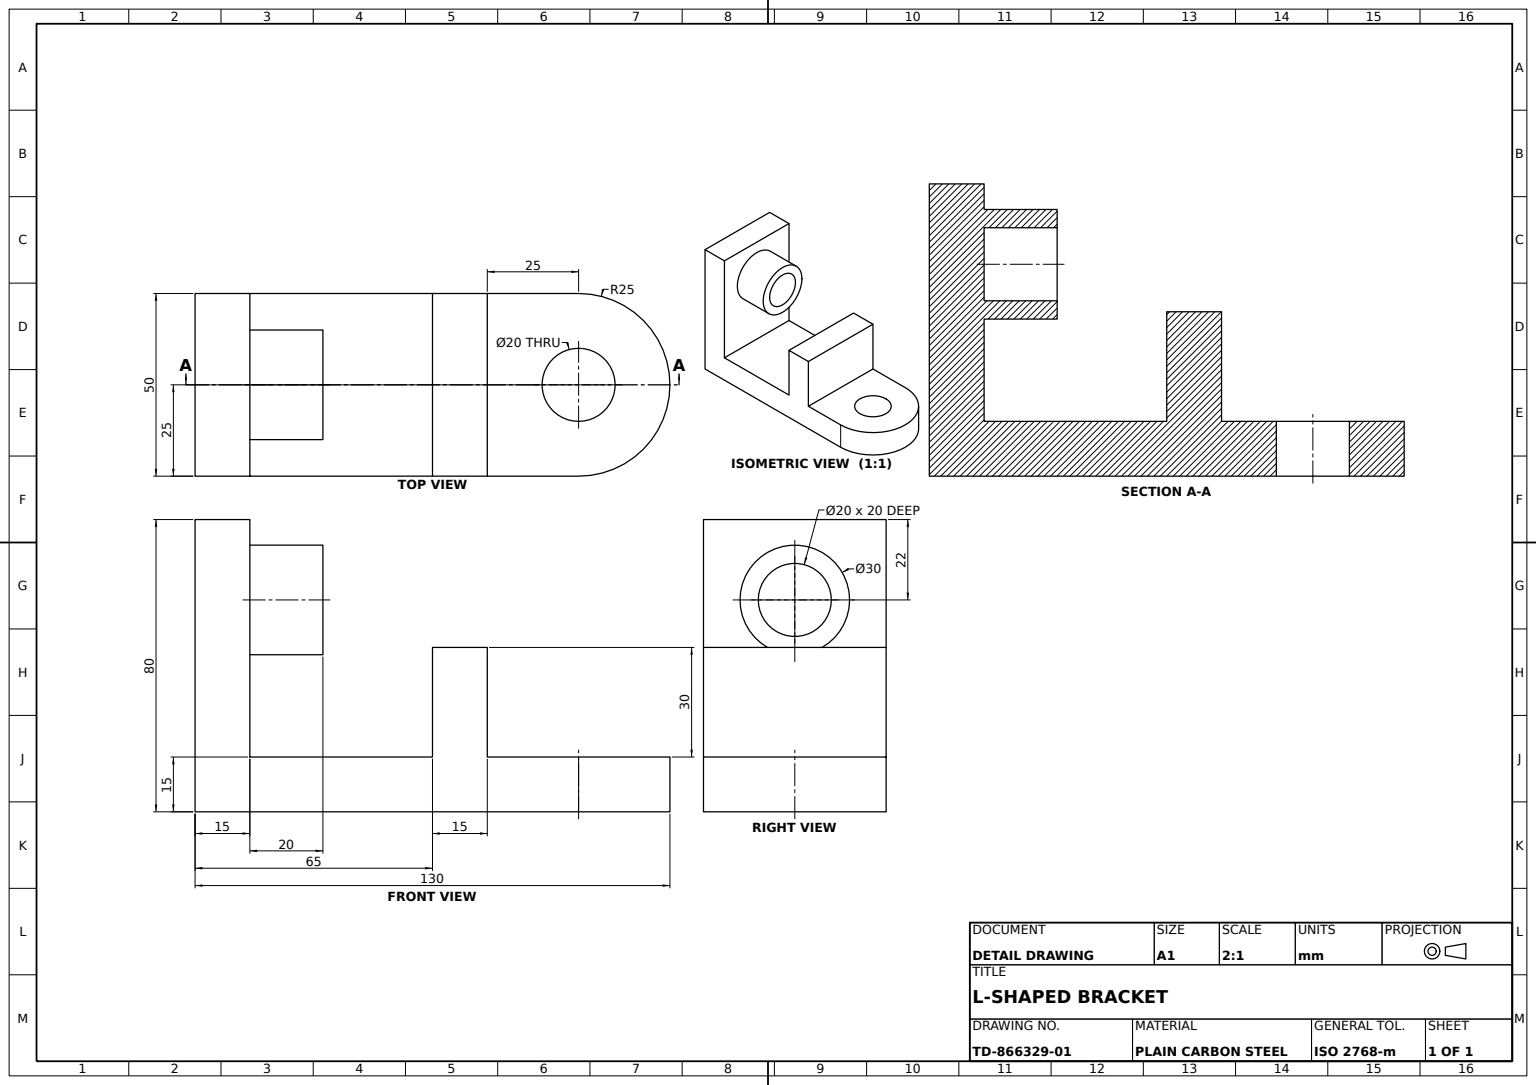
SolidWorks part; units mm, degrees
material "Plain Carbon Steel"
ref_plane "Front Plane" through (0, 0, 0) normal (0, 0, 1) x (1, 0, 0)
ref_plane "Top Plane" through (0, 0, 0) normal (0, 1, 0) x (1, 0, 0)
ref_plane "Right Plane" through (0, 0, 0) normal (1, 0, 0) x (0, 0, -1)
sketch "Base Plate Sketch" plane through (0, 0, 0) normal (0, 1, 0) x (1, 0, 0)
  line L1 (-65, -25) -> (40, -25)
  line L2 (-65, -25) -> (-65, 25)
  line L3 (-65, 25) -> (40, 25)
  arc A0 (40, -25) -> (40, 25) centre (40, 0) ccw
  point P0 (0, 0)
  point P1 (-65, 0)
  point P4 (65, 0)
  dimension "D3" = 25
  dimension "D4" = 25
  dimension "D1" = 130
  dimension "D2" = 50
  dimension "D5" = 65
extrude "Base Plate" add sketch "Base Plate Sketch" along normal blind 15
sketch "Upright Wall Sketch" plane through (0, 15, 0) normal (0, 1, 0) x (1, 0, 0)
  line L0 (40, 25) -> (-65, 25) construction
  line L1 (-65, -25) -> (-50, -25)
  line L2 (-65, -25) -> (-65, 25)
  line L3 (-65, 25) -> (-50, 25)
  line L4 (-50, -25) -> (-50, 25)
  dimension "D1" = 15
extrude "Upright Wall" add sketch "Upright Wall Sketch" along normal blind 65
sketch "Wall Boss Sketch" plane through (-50, 0, 0) normal (1, 0, 0) x (0, 0, -1)
  line L0 (-25, 80) -> (25, 80) construction
  line L2 (-25, 80) -> (-25, 15) construction
  circle A0 centre (0, 58) radius 15
  dimension "D1" = 15
  dimension "D2" = 22
  dimension "D3" = 25
extrude "Wall Boss" add sketch "Wall Boss Sketch" along normal blind 20
sketch "Boss Bore Sketch" plane through (-30, 0, 0) normal (1, 0, 0) x (0, 0, -1)
  circle A0 centre (0, 58) radius 10
  dimension "D1" = 10
extrude "Boss Bore Ø10" cut sketch "Boss Bore Sketch" against normal blind 20
sketch "Raised Block Sketch" plane through (0, 15, 0) normal (0, 1, 0) x (1, 0, 0)
  line L0 (15, 25) -> (15, -25)
  line L1 (40, 25) -> (-50, 25) construction
  line L2 (-50, -25) -> (40, -25) construction
  line L3 (15, -25) -> (0, -25)
  line L4 (0, -25) -> (0, 25)
  line L5 (0, 25) -> (15, 25)
  line L6 (0, 0) -> (65, 0) construction
  arc A0 (40, -25) -> (40, 25) centre (40, 0) ccw construction
  point P14 (15, 0)
  dimension "D1" = 50
extrude "Raised Block" add sketch "Raised Block Sketch" along normal blind 30
sketch "Lug Hole Sketch" plane through (0, 15, 0) normal (0, 1, 0) x (1, 0, 0)
  line L0 (40, 25) -> (40, -25) construction
  arc A0 (40, -25) -> (40, 25) centre (40, 0) ccw construction
  circle A1 centre (40, 0) radius 10
  dimension "D1" = 10
extrude "Lug Hole" cut sketch "Lug Hole Sketch" against normal blind 15
